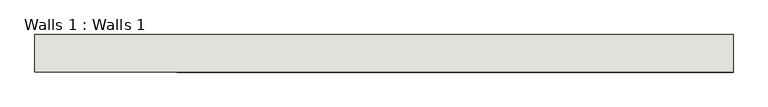
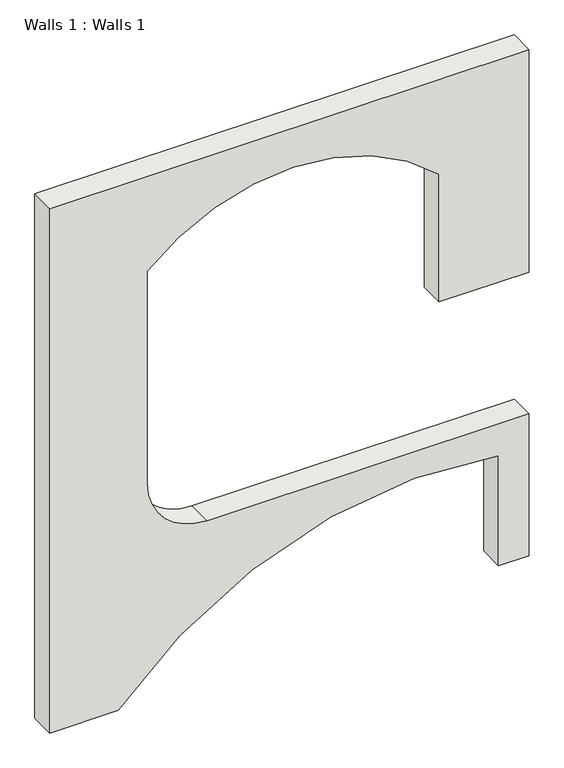
"""IFC4 building model written with IfcOpenShell, lengths in millimetres: wall geometry, Walls 1 : Walls 1."""

from ifc_helpers import new_model, si_unit, point, frame, frame_2d, origin, place, context, project, spatial, polyline, circle_curve, trimmed, segment, composite_curve, outline, extrude, source, transform, mapped, element, save


def walls_1_walls_1_8e9adab5(model_context):
    return source(origin(), model_context, "Body", "SweptSolid", [
        extrude(outline(composite_curve([segment(polyline([(13925.6, -9031.8352527), (2648.0, -9031.8352527), (2648.0, -7641.5935835)]), True, "CONTINUOUS"), segment(trimmed(circle_curve(frame_2d((-2863.3221432, -1306.0790316)), 8397.2267091), [point((2648.0, -7641.5935835))], [point((5415.0926692, 101.4949802))], True, "CARTESIAN"), True, "CONTINUOUS"), segment(polyline([(5415.0926692, 101.4949802), (3048.0, 101.4949802), (3048.0, 721.7647473), (6096.0, 721.7647473), (6096.0, -5831.4352527)]), True, "CONTINUOUS"), segment(trimmed(circle_curve(frame_2d((7315.2, -5831.4352527)), 1219.2), [point((6096.0, -5831.4352527))], [point((7315.2, -7050.6352527))], True, "CARTESIAN"), True, "CONTINUOUS"), segment(polyline([(7315.2, -7050.6352527), (11887.2, -7050.6352527)]), True, "CONTINUOUS"), segment(trimmed(circle_curve(frame_2d((8760.2968069, -4078.8352527)), 4313.8287888), [point((11887.2, -7050.6352527))], [point((11887.2, -1107.0352527))], True, "CARTESIAN"), True, "CONTINUOUS"), segment(polyline([(11887.2, -1107.0352527), (9144.0, -1107.0352527), (9144.0, 721.7647473), (13925.6, 721.7647473), (13925.6, -9031.8352527)]), True, "CONTINUOUS")], self_intersect=False)), frame((0.0, -1113.4287891, 0.0), z_axis=(0.0, 1.0, 0.0), x_axis=(0.0, 0.0, 1.0)), (0.0, 0.0, 1.0), 524.2436336),
    ])


if __name__ == "__main__":
    model = new_model("IFC4")
    model_context = context("Model", 3, world=origin())
    ifc_project = project(units=[si_unit("LENGTHUNIT", "METRE", prefix="MILLI")], contexts=[model_context])
    site = spatial("IfcSite", under=ifc_project)
    building = spatial("IfcBuilding", under=site)
    placement = place(None, origin())
    walls_1_walls_1_shape = walls_1_walls_1_8e9adab5(model_context)
    element("IfcWall", 1, ObjectType="Walls 1 : Walls 1", at=placement, inside=building, context=model_context, shape_type="MappedRepresentation", body=[
        mapped(walls_1_walls_1_shape, transform((0.0, 0.0, 0.0), x_axis=(1.0, 0.0, 0.0), y_axis=(0.0, 1.0, 0.0), z_axis=(0.0, 0.0, 1.0))),
    ])
    save(model, "model.ifc")

# Revit data of these elements
# Element 1 (IfcWall, "Walls 1 : Walls 1")
#   Materials on its faces: "Default Wall"
# Materials
#   "Default Wall": colour RGB 80 80 80, transparency 0
